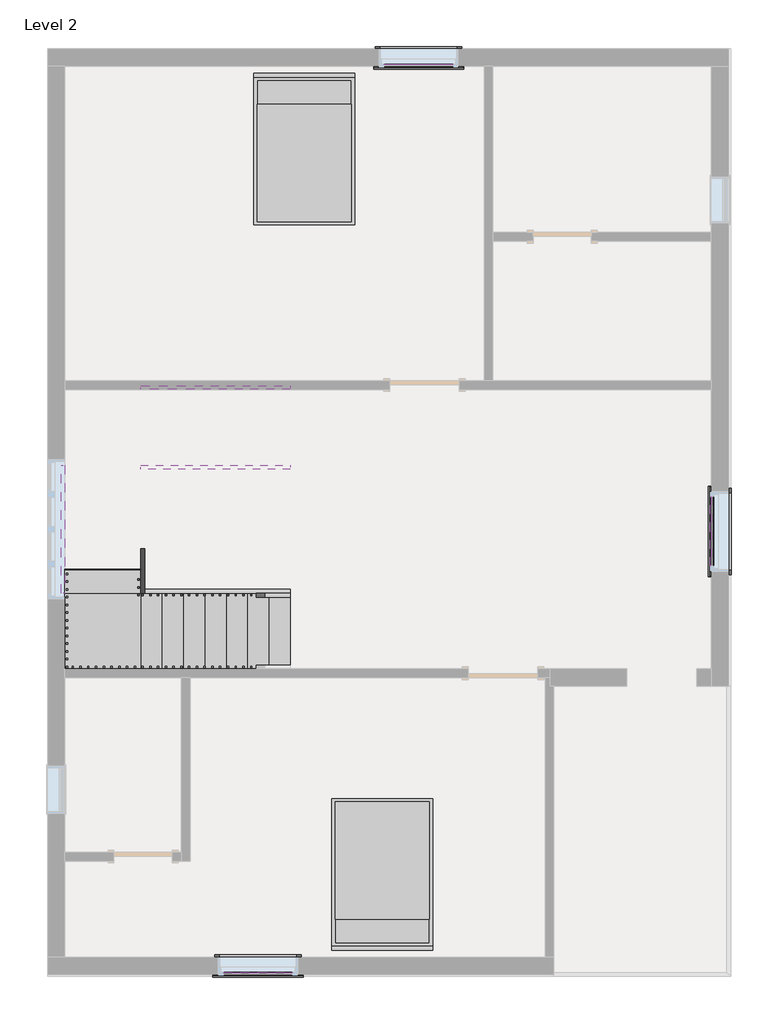
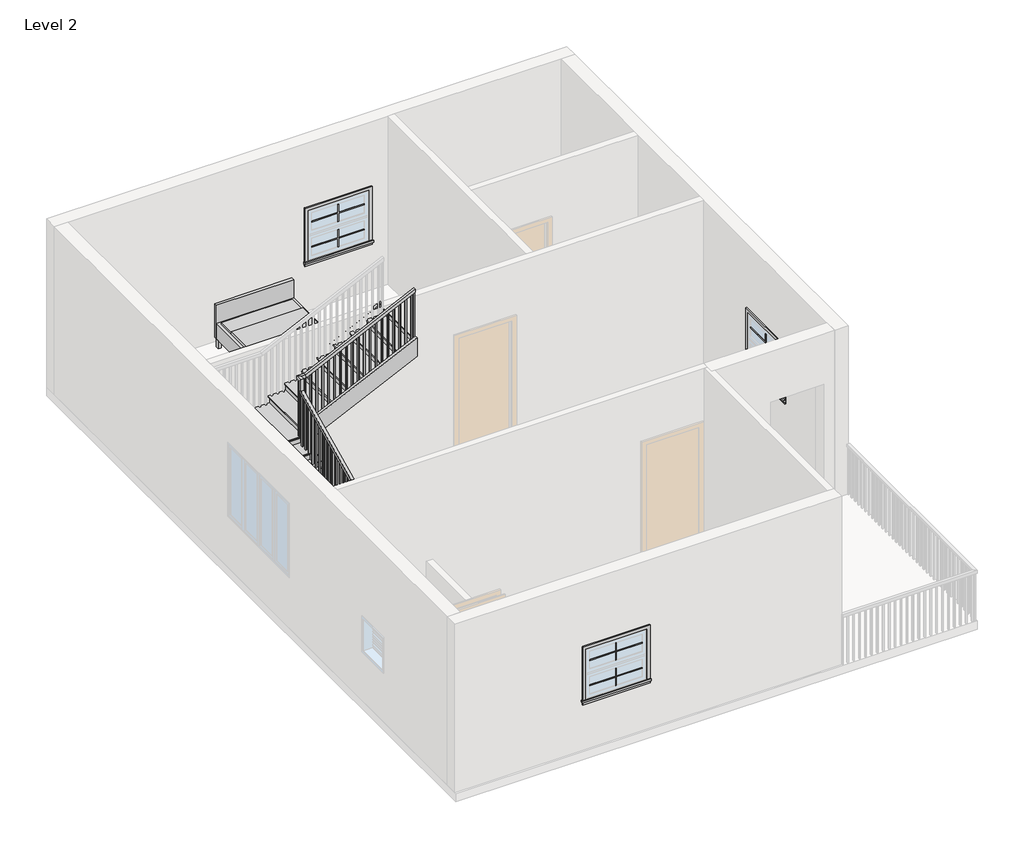
# One storey, part 3 of 3: 12 proxies, 6 members, 2 furniture elements, 1 railing, 1 stair flight.
"""IFC4 building model written with IfcOpenShell, lengths in millimetres."""

from ifc_helpers import new_model, si_unit, frame, origin, place, context, project, spatial, polyline, outline, extrude, faceted_brep, transform, mapped, element, save
from components import muntin_pattern_2x2_muntin_pattern_2x2_4e6d5dbc, muntin_pattern_2x2_muntin_pattern_2x2_9ec9cf3e, trim_window_exterior_flat_with_sill_79aa6636, trim_window_interior_flat_picture_frame_55a9d760, bed_17739_bed_17739_15c61121, stair_flight_9d362d5c

model = new_model("IFC4")

# Units and contexts
model_context = context("Model", 3, world=origin())
ifc_project = project(units=[si_unit("LENGTHUNIT", "METRE", prefix="MILLI")], contexts=[model_context])

# Site, building, storey
site = spatial("IfcSite", under=ifc_project)
building = spatial("IfcBuilding", under=site)
storey = spatial("IfcBuildingStorey", under=building, Name="Level 2", Elevation=3048.0)

# Proxies
placement = place(None, origin())
muntin_pattern_2x2_muntin_pattern_2x2_shape = muntin_pattern_2x2_muntin_pattern_2x2_4e6d5dbc(model_context)
element("IfcBuildingElementProxy", 1, Name="Muntin Pattern_2x2 : Muntin Pattern_2x2", ObjectType="Muntin Pattern_2x2 : Muntin Pattern_2x2", at=placement, inside=storey, context=model_context, shape_type="MappedRepresentation", body=[
    mapped(muntin_pattern_2x2_muntin_pattern_2x2_shape, transform((-20188.9789184, -5109.4149287, 4489.45), x_axis=(-1.0, 0.0, 0.0), y_axis=(0.0, -1.0, 0.0), z_axis=(0.0, 0.0, 1.0))),
])
element("IfcBuildingElementProxy", 2, Name="Muntin Pattern_2x2 : Muntin Pattern_2x2", ObjectType="Muntin Pattern_2x2 : Muntin Pattern_2x2", at=placement, inside=storey, context=model_context, shape_type="MappedRepresentation", body=[
    mapped(muntin_pattern_2x2_muntin_pattern_2x2_shape, transform((-14248.5539184, 681.7850713, 4489.45), x_axis=(0.0, 1.0, 0.0), y_axis=(-1.0, 0.0, 0.0), z_axis=(0.0, 0.0, 1.0))),
])
element("IfcBuildingElementProxy", 3, Name="Muntin Pattern_2x2 : Muntin Pattern_2x2", ObjectType="Muntin Pattern_2x2 : Muntin Pattern_2x2", at=placement, inside=storey, context=model_context, shape_type="MappedRepresentation", body=[
    mapped(muntin_pattern_2x2_muntin_pattern_2x2_shape, transform((-18087.1289184, 6777.7850713, 4489.45), x_axis=(-1.0, 0.0, 0.0), y_axis=(0.0, -1.0, 0.0), z_axis=(0.0, 0.0, 1.0))),
])
muntin_pattern_2x2_muntin_pattern_2x2_2_shape = muntin_pattern_2x2_muntin_pattern_2x2_9ec9cf3e(model_context)
element("IfcBuildingElementProxy", 4, Name="Muntin Pattern_2x2 : Muntin Pattern_2x2", ObjectType="Muntin Pattern_2x2 : Muntin Pattern_2x2", at=placement, inside=storey, context=model_context, shape_type="MappedRepresentation", body=[
    mapped(muntin_pattern_2x2_muntin_pattern_2x2_2_shape, transform((-20188.9789184, -5109.4149287, 4032.25), x_axis=(-1.0, 0.0, 0.0), y_axis=(0.0, -1.0, 0.0), z_axis=(0.0, 0.0, 1.0))),
])
element("IfcBuildingElementProxy", 5, Name="Muntin Pattern_2x2 : Muntin Pattern_2x2", ObjectType="Muntin Pattern_2x2 : Muntin Pattern_2x2", at=placement, inside=storey, context=model_context, shape_type="MappedRepresentation", body=[
    mapped(muntin_pattern_2x2_muntin_pattern_2x2_2_shape, transform((-14248.5539184, 681.7850713, 4032.25), x_axis=(0.0, 1.0, 0.0), y_axis=(-1.0, 0.0, 0.0), z_axis=(0.0, 0.0, 1.0))),
])
element("IfcBuildingElementProxy", 6, Name="Muntin Pattern_2x2 : Muntin Pattern_2x2", ObjectType="Muntin Pattern_2x2 : Muntin Pattern_2x2", at=placement, inside=storey, context=model_context, shape_type="MappedRepresentation", body=[
    mapped(muntin_pattern_2x2_muntin_pattern_2x2_2_shape, transform((-18087.1289184, 6777.7850713, 4032.25), x_axis=(-1.0, 0.0, 0.0), y_axis=(0.0, -1.0, 0.0), z_axis=(0.0, 0.0, 1.0))),
])
trim_window_exterior_flat_with_sill_shape = trim_window_exterior_flat_with_sill_79aa6636(model_context)
element("IfcBuildingElementProxy", 7, Name="Trim-Window-Exterior-Flat : with Sill", ObjectType="Trim-Window-Exterior-Flat : with Sill", at=placement, inside=storey, context=model_context, shape_type="MappedRepresentation", body=[
    mapped(trim_window_exterior_flat_with_sill_shape, transform((-20188.9789184, -5118.9399287, 4876.8), x_axis=(1.0, 0.0, 0.0), y_axis=(0.0, 0.0, 1.0), z_axis=(0.0, -1.0, 0.0))),
])
element("IfcBuildingElementProxy", 8, Name="Trim-Window-Exterior-Flat : with Sill", ObjectType="Trim-Window-Exterior-Flat : with Sill", at=placement, inside=storey, context=model_context, shape_type="MappedRepresentation", body=[
    mapped(trim_window_exterior_flat_with_sill_shape, transform((-14258.0789184, 681.7850713, 4876.8), x_axis=(0.0, -1.0, 0.0), y_axis=(0.0, 0.0, 1.0), z_axis=(-1.0, 0.0, 0.0))),
])
element("IfcBuildingElementProxy", 9, Name="Trim-Window-Exterior-Flat : with Sill", ObjectType="Trim-Window-Exterior-Flat : with Sill", at=placement, inside=storey, context=model_context, shape_type="MappedRepresentation", body=[
    mapped(trim_window_exterior_flat_with_sill_shape, transform((-18087.1289184, 6768.2600713, 4876.8), x_axis=(1.0, 0.0, 0.0), y_axis=(0.0, 0.0, 1.0), z_axis=(0.0, -1.0, 0.0))),
])
trim_window_interior_flat_picture_frame_shape = trim_window_interior_flat_picture_frame_55a9d760(model_context)
element("IfcBuildingElementProxy", 10, Name="Trim-Window-Interior-Flat : Picture Frame", ObjectType="Trim-Window-Interior-Flat : Picture Frame", at=placement, inside=storey, context=model_context, shape_type="MappedRepresentation", body=[
    mapped(trim_window_interior_flat_picture_frame_shape, transform((-20188.9789184, -4890.3399287, 4876.8), x_axis=(-1.0, 0.0, 0.0), y_axis=(0.0, 0.0, 1.0), z_axis=(0.0, 1.0, 0.0))),
])
element("IfcBuildingElementProxy", 11, Name="Trim-Window-Interior-Flat : Picture Frame", ObjectType="Trim-Window-Interior-Flat : Picture Frame", at=placement, inside=storey, context=model_context, shape_type="MappedRepresentation", body=[
    mapped(trim_window_interior_flat_picture_frame_shape, transform((-14029.4789184, 681.7850713, 4876.8), x_axis=(0.0, 1.0, 0.0), y_axis=(0.0, 0.0, 1.0), z_axis=(1.0, 0.0, 0.0))),
])
element("IfcBuildingElementProxy", 12, Name="Trim-Window-Interior-Flat : Picture Frame", ObjectType="Trim-Window-Interior-Flat : Picture Frame", at=placement, inside=storey, context=model_context, shape_type="MappedRepresentation", body=[
    mapped(trim_window_interior_flat_picture_frame_shape, transform((-18087.1289184, 6996.8600713, 4876.8), x_axis=(-1.0, 0.0, 0.0), y_axis=(0.0, 0.0, 1.0), z_axis=(0.0, 1.0, 0.0))),
])

# Furniture
bed_17739_bed_17739_shape = bed_17739_bed_17739_15c61121(model_context)
element("IfcFurniture", 13, ObjectType="Bed_17739 : Bed_17739", at=placement, inside=storey, context=model_context, shape_type="MappedRepresentation", body=[
    mapped(bed_17739_bed_17739_shape, transform((-18563.3789184, -3785.4399287, 3048.0), x_axis=(-1.0, 0.0, 0.0), y_axis=(0.0, -1.0, 0.0), z_axis=(0.0, 0.0, 1.0))),
])
element("IfcFurniture", 14, ObjectType="Bed_17739 : Bed_17739", at=placement, inside=storey, context=model_context, shape_type="MappedRepresentation", body=[
    mapped(bed_17739_bed_17739_shape, transform((-19585.7289184, 5663.3600713, 3048.0), x_axis=(1.0, 0.0, 0.0), y_axis=(0.0, 1.0, 0.0), z_axis=(0.0, 0.0, 1.0))),
])

# Members
element("IfcMember", 15, ObjectType="Stringer - 2\" Width", at=placement, inside=storey, context=model_context, shape_type="SweptSolid", body=[
    extrude(outline(polyline([(3048.0, -19769.8789184), (3249.2074226, -19769.8789184), (3839.5315333, -21014.4789184), (3839.5315333, -21725.7197387), (3048.0, -20056.9074227), (3048.0, -19769.8789184)])), frame((0.0, -1169.2399287, 0.0), z_axis=(0.0, 1.0, 0.0), x_axis=(0.0, 0.0, 1.0)), (0.0, 0.0, 1.0), 50.8),
])
element("IfcMember", 16, ObjectType="Stringer - 2\" Width", at=placement, inside=storey, context=model_context, shape_type="SweptSolid", body=[
    extrude(outline(polyline([(-127.880749, 4309.3619743), (837.3600713, 4767.1837072), (1548.6008915, 4767.1837072), (583.3600713, 4309.3619743), (-127.880749, 4309.3619743)])), frame((-22767.0789184, 0.0, 0.0), z_axis=(1.0, 0.0, 0.0), x_axis=(0.0, 1.0, 0.0)), (0.0, 0.0, 1.0), 50.8),
])
element("IfcMember", 17, ObjectType="Stringer - 2\" Width", at=placement, inside=storey, context=model_context, shape_type="SweptSolid", body=[
    extrude(outline(polyline([(5237.0141482, -21014.4789184), (5827.3382589, -19769.8789184), (6164.6856835, -19769.8789184), (5237.0141482, -21725.7197387), (5237.0141482, -21014.4789184)])), frame((0.0, 2539.1600713, 0.0), z_axis=(0.0, 1.0, 0.0), x_axis=(0.0, 0.0, 1.0)), (0.0, 0.0, 1.0), 50.8),
])
element("IfcMember", 18, ObjectType="Stringer - 2\" Width", at=placement, inside=storey, context=model_context, shape_type="SweptSolid", body=[
    extrude(outline(polyline([(3048.0, -19769.8789184), (3249.2074226, -19769.8789184), (4152.7647349, -21674.8789184), (3815.4173103, -21674.8789184), (3048.0, -20056.9074227), (3048.0, -19769.8789184)])), frame((0.0, -127.8399287, 0.0), z_axis=(0.0, 1.0, 0.0), x_axis=(0.0, 0.0, 1.0)), (0.0, 0.0, 1.0), 50.8),
])
element("IfcMember", 19, ObjectType="Stringer - 2\" Width", at=placement, inside=storey, context=model_context, shape_type="SweptSolid", body=[
    extrude(outline(polyline([(-127.8399287, 3972.033911), (-127.8399287, 4309.3813357), (1497.7600713, 5080.4169088), (1497.7600713, 4743.0694842), (-127.8399287, 3972.033911)])), frame((-21725.6789184, 0.0, 0.0), z_axis=(1.0, 0.0, 0.0), x_axis=(0.0, 1.0, 0.0)), (0.0, 0.0, 1.0), 50.8),
])
element("IfcMember", 20, ObjectType="Stringer - 2\" Width", at=placement, inside=storey, context=model_context, shape_type="SweptSolid", body=[
    extrude(outline(polyline([(5237.0335096, -21725.6789184), (4899.686085, -21725.6789184), (5827.3382589, -19769.8789184), (6164.6856835, -19769.8789184), (5237.0335096, -21725.6789184)])), frame((0.0, 1497.7600713, 0.0), z_axis=(0.0, 1.0, 0.0), x_axis=(0.0, 0.0, 1.0)), (0.0, 0.0, 1.0), 50.8),
])

# Railing
element("IfcRailing", 21, ObjectType="Handrail - Rectangular", at=placement, inside=storey, context=model_context, shape_type="SolidModel", body=[
    faceted_brep([(-19769.8789184, -178.6399287, 4094.9217391), (-19769.8789184, -178.6399287, 4038.6971684), (-19769.8789184, -127.8399287, 4038.6971684), (-19769.8789184, -127.8399287, 4094.9217391), (-21649.4789184, -178.6399287, 4986.4316206), (-21700.2789184, -178.6399287, 4954.3019114), (-21700.2789184, -127.8399287, 4954.3019114), (-21649.4789184, -127.8399287, 4986.4316206), (-21776.4789184, -40.2031254, 5140.4379447), (-21776.4789184, -51.6399287, 5191.2379447), (-21776.4789184, 1472.3600713, 5914.0837945), (-21776.4789184, 1523.1600713, 5881.9540854), (-21725.6789184, -40.2031254, 5140.4379447), (-21725.6789184, 1523.1600713, 5881.9540854), (-21725.6789184, -51.6399287, 5191.2379447), (-21725.6789184, 1472.3600713, 5914.0837945), (-19769.8789184, 1599.3600713, 7010.4), (-19769.8789184, 1548.5600713, 7010.4), (-19769.8789184, 1548.5600713, 6954.1754292), (-19769.8789184, 1599.3600713, 6954.1754292), (-21638.0421151, 1599.3600713, 6068.0901186), (-21649.4789184, 1599.3600713, 6118.8901186), (-21638.0421151, 1548.5600713, 6068.0901186), (-21649.4789184, 1548.5600713, 6118.8901186), (-21649.4789184, -178.6399287, 5191.2379447), (-21700.2789184, -178.6399287, 5140.4379447), (-21700.2789184, -127.8399287, 5140.4379447), (-21649.4789184, -127.8399287, 5191.2379447), (-21776.4789184, -178.6399287, 5191.2379447), (-21776.4789184, -178.6399287, 5140.4379447), (-21725.6789184, -127.8399287, 5140.4379447), (-21725.6789184, -127.8399287, 5191.2379447), (-21776.4789184, 1472.3600713, 6118.8901186), (-21776.4789184, 1523.1600713, 6068.0901186), (-21725.6789184, 1523.1600713, 6068.0901186), (-21725.6789184, 1472.3600713, 6118.8901186), (-21776.4789184, 1599.3600713, 6118.8901186), (-21776.4789184, 1599.3600713, 6068.0901186), (-21725.6789184, 1548.5600713, 6068.0901186), (-21725.6789184, 1548.5600713, 6118.8901186)], [[[0, 1, 2, 3]], [[1, 0, 4, 5]], [[2, 1, 5, 6]], [[3, 2, 6, 7]], [[0, 3, 7, 4]], [[8, 9, 10, 11]], [[12, 8, 11, 13]], [[14, 12, 13, 15]], [[9, 14, 15, 10]], [[16, 17, 18, 19]], [[20, 21, 16, 19]], [[22, 20, 19, 18]], [[23, 22, 18, 17]], [[21, 23, 17, 16]], [[5, 4, 24, 25]], [[6, 5, 25, 26]], [[7, 6, 26, 27]], [[4, 7, 27, 24]], [[25, 24, 28, 29]], [[26, 25, 29, 30]], [[27, 26, 30, 31]], [[24, 27, 31, 28]], [[29, 28, 9, 8]], [[30, 29, 8, 12]], [[31, 30, 12, 14]], [[28, 31, 14, 9]], [[11, 10, 32, 33]], [[13, 11, 33, 34]], [[15, 13, 34, 35]], [[10, 15, 35, 32]], [[33, 32, 36, 37]], [[34, 33, 37, 38]], [[35, 34, 38, 39]], [[32, 35, 39, 36]], [[37, 36, 21, 20]], [[38, 37, 20, 22]], [[39, 38, 22, 23]], [[36, 39, 23, 21]]]),
    extrude(outline(polyline([(6934.5983541, -19811.1539184), (6925.562781, -19830.2039184), (5963.4782609, -19830.2039184), (5963.4782609, -19811.1539184), (6934.5983541, -19811.1539184)])), frame((0.0, 1564.4350713, 0.0), z_axis=(0.0, 1.0, 0.0), x_axis=(0.0, 0.0, 1.0)), (0.0, 0.0, 1.0), 19.05),
    extrude(outline(polyline([(6886.4086308, -19912.7539184), (6877.3730577, -19931.8039184), (5963.4782609, -19931.8039184), (5963.4782609, -19912.7539184), (6886.4086308, -19912.7539184)])), frame((0.0, 1564.4350713, 0.0), z_axis=(0.0, 1.0, 0.0), x_axis=(0.0, 0.0, 1.0)), (0.0, 0.0, 1.0), 19.05),
    extrude(outline(polyline([(6838.2189075, -20014.3539184), (6829.1833344, -20033.4039184), (5963.4782609, -20033.4039184), (5963.4782609, -20014.3539184), (6838.2189075, -20014.3539184)])), frame((0.0, 1564.4350713, 0.0), z_axis=(0.0, 1.0, 0.0), x_axis=(0.0, 0.0, 1.0)), (0.0, 0.0, 1.0), 19.05),
    extrude(outline(polyline([(6790.0291842, -20115.9539184), (6780.993611, -20135.0039184), (5830.9565217, -20135.0039184), (5830.9565217, -20115.9539184), (6790.0291842, -20115.9539184)])), frame((0.0, 1564.4350713, 0.0), z_axis=(0.0, 1.0, 0.0), x_axis=(0.0, 0.0, 1.0)), (0.0, 0.0, 1.0), 19.05),
    extrude(outline(polyline([(6741.8394608, -20217.5539184), (6732.8038877, -20236.6039184), (5830.9565217, -20236.6039184), (5830.9565217, -20217.5539184), (6741.8394608, -20217.5539184)])), frame((0.0, 1564.4350713, 0.0), z_axis=(0.0, 1.0, 0.0), x_axis=(0.0, 0.0, 1.0)), (0.0, 0.0, 1.0), 19.05),
    extrude(outline(polyline([(6693.6497375, -20319.1539184), (6684.6141644, -20338.2039184), (5830.9565217, -20338.2039184), (5830.9565217, -20319.1539184), (6693.6497375, -20319.1539184)])), frame((0.0, 1564.4350713, 0.0), z_axis=(0.0, 1.0, 0.0), x_axis=(0.0, 0.0, 1.0)), (0.0, 0.0, 1.0), 19.05),
    extrude(outline(polyline([(6645.4600142, -20420.7539184), (6636.4244411, -20439.8039184), (5698.4347826, -20439.8039184), (5698.4347826, -20420.7539184), (6645.4600142, -20420.7539184)])), frame((0.0, 1564.4350713, 0.0), z_axis=(0.0, 1.0, 0.0), x_axis=(0.0, 0.0, 1.0)), (0.0, 0.0, 1.0), 19.05),
    extrude(outline(polyline([(6597.2702909, -20522.3539184), (6588.2347178, -20541.4039184), (5698.4347826, -20541.4039184), (5698.4347826, -20522.3539184), (6597.2702909, -20522.3539184)])), frame((0.0, 1564.4350713, 0.0), z_axis=(0.0, 1.0, 0.0), x_axis=(0.0, 0.0, 1.0)), (0.0, 0.0, 1.0), 19.05),
    extrude(outline(polyline([(6549.0805676, -20623.9539184), (6540.0449944, -20643.0039184), (5565.9130435, -20643.0039184), (5565.9130435, -20623.9539184), (6549.0805676, -20623.9539184)])), frame((0.0, 1564.4350713, 0.0), z_axis=(0.0, 1.0, 0.0), x_axis=(0.0, 0.0, 1.0)), (0.0, 0.0, 1.0), 19.05),
    extrude(outline(polyline([(6500.8908442, -20725.5539184), (6491.8552711, -20744.6039184), (5565.9130435, -20744.6039184), (5565.9130435, -20725.5539184), (6500.8908442, -20725.5539184)])), frame((0.0, 1564.4350713, 0.0), z_axis=(0.0, 1.0, 0.0), x_axis=(0.0, 0.0, 1.0)), (0.0, 0.0, 1.0), 19.05),
    extrude(outline(polyline([(6452.7011209, -20827.1539184), (6443.6655478, -20846.2039184), (5565.9130435, -20846.2039184), (5565.9130435, -20827.1539184), (6452.7011209, -20827.1539184)])), frame((0.0, 1564.4350713, 0.0), z_axis=(0.0, 1.0, 0.0), x_axis=(0.0, 0.0, 1.0)), (0.0, 0.0, 1.0), 19.05),
    extrude(outline(polyline([(6404.5113976, -20928.7539184), (6395.4758245, -20947.8039184), (5433.3913043, -20947.8039184), (5433.3913043, -20928.7539184), (6404.5113976, -20928.7539184)])), frame((0.0, 1564.4350713, 0.0), z_axis=(0.0, 1.0, 0.0), x_axis=(0.0, 0.0, 1.0)), (0.0, 0.0, 1.0), 19.05),
    extrude(outline(polyline([(6356.3216743, -21030.3539184), (6347.2861012, -21049.4039184), (5433.3913043, -21049.4039184), (5433.3913043, -21030.3539184), (6356.3216743, -21030.3539184)])), frame((0.0, 1564.4350713, 0.0), z_axis=(0.0, 1.0, 0.0), x_axis=(0.0, 0.0, 1.0)), (0.0, 0.0, 1.0), 19.05),
    extrude(outline(polyline([(6308.131951, -21131.9539184), (6299.0963778, -21151.0039184), (5433.3913043, -21151.0039184), (5433.3913043, -21131.9539184), (6308.131951, -21131.9539184)])), frame((0.0, 1564.4350713, 0.0), z_axis=(0.0, 1.0, 0.0), x_axis=(0.0, 0.0, 1.0)), (0.0, 0.0, 1.0), 19.05),
    extrude(outline(polyline([(6259.9422276, -21233.5539184), (6250.9066545, -21252.6039184), (5300.8695652, -21252.6039184), (5300.8695652, -21233.5539184), (6259.9422276, -21233.5539184)])), frame((0.0, 1564.4350713, 0.0), z_axis=(0.0, 1.0, 0.0), x_axis=(0.0, 0.0, 1.0)), (0.0, 0.0, 1.0), 19.05),
    extrude(outline(polyline([(6211.7525043, -21335.1539184), (6202.7169312, -21354.2039184), (5300.8695652, -21354.2039184), (5300.8695652, -21335.1539184), (6211.7525043, -21335.1539184)])), frame((0.0, 1564.4350713, 0.0), z_axis=(0.0, 1.0, 0.0), x_axis=(0.0, 0.0, 1.0)), (0.0, 0.0, 1.0), 19.05),
    extrude(outline(polyline([(6163.562781, -21436.7539184), (6154.5272079, -21455.8039184), (5300.8695652, -21455.8039184), (5300.8695652, -21436.7539184), (6163.562781, -21436.7539184)])), frame((0.0, 1564.4350713, 0.0), z_axis=(0.0, 1.0, 0.0), x_axis=(0.0, 0.0, 1.0)), (0.0, 0.0, 1.0), 19.05),
    extrude(outline(polyline([(6115.3730577, -21538.3539184), (6106.3374846, -21557.4039184), (5168.3478261, -21557.4039184), (5168.3478261, -21538.3539184), (6115.3730577, -21538.3539184)])), frame((0.0, 1564.4350713, 0.0), z_axis=(0.0, 1.0, 0.0), x_axis=(0.0, 0.0, 1.0)), (0.0, 0.0, 1.0), 19.05),
    extrude(outline(polyline([(6067.1833344, -21639.9539184), (6058.1477612, -21659.0039184), (5168.3478261, -21659.0039184), (5168.3478261, -21639.9539184), (6067.1833344, -21639.9539184)])), frame((0.0, 1564.4350713, 0.0), z_axis=(0.0, 1.0, 0.0), x_axis=(0.0, 0.0, 1.0)), (0.0, 0.0, 1.0), 19.05),
    extrude(outline(polyline([(1462.8350713, 5853.3414371), (1481.8850713, 5862.3770103), (1481.8850713, 4903.3043478), (1462.8350713, 4903.3043478), (1462.8350713, 5853.3414371)])), frame((-21760.6039184, 0.0, 0.0), z_axis=(1.0, 0.0, 0.0), x_axis=(0.0, 1.0, 0.0)), (0.0, 0.0, 1.0), 19.05),
    extrude(outline(polyline([(1361.2350713, 5805.1517138), (1380.2850713, 5814.1872869), (1380.2850713, 4903.3043478), (1361.2350713, 4903.3043478), (1361.2350713, 5805.1517138)])), frame((-21760.6039184, 0.0, 0.0), z_axis=(1.0, 0.0, 0.0), x_axis=(0.0, 1.0, 0.0)), (0.0, 0.0, 1.0), 19.05),
    extrude(outline(polyline([(1259.6350713, 5756.9619905), (1278.6850713, 5765.9975636), (1278.6850713, 4903.3043478), (1259.6350713, 4903.3043478), (1259.6350713, 5756.9619905)])), frame((-21760.6039184, 0.0, 0.0), z_axis=(1.0, 0.0, 0.0), x_axis=(0.0, 1.0, 0.0)), (0.0, 0.0, 1.0), 19.05),
    extrude(outline(polyline([(1158.0350713, 5708.7722672), (1177.0850713, 5717.8078403), (1177.0850713, 4770.7826087), (1158.0350713, 4770.7826087), (1158.0350713, 5708.7722672)])), frame((-21760.6039184, 0.0, 0.0), z_axis=(1.0, 0.0, 0.0), x_axis=(0.0, 1.0, 0.0)), (0.0, 0.0, 1.0), 19.05),
    extrude(outline(polyline([(1056.4350713, 5660.5825439), (1075.4850713, 5669.618117), (1075.4850713, 4770.7826087), (1056.4350713, 4770.7826087), (1056.4350713, 5660.5825439)])), frame((-21760.6039184, 0.0, 0.0), z_axis=(1.0, 0.0, 0.0), x_axis=(0.0, 1.0, 0.0)), (0.0, 0.0, 1.0), 19.05),
    extrude(outline(polyline([(954.8350713, 5612.3928205), (973.8850713, 5621.4283937), (973.8850713, 4638.2608696), (954.8350713, 4638.2608696), (954.8350713, 5612.3928205)])), frame((-21760.6039184, 0.0, 0.0), z_axis=(1.0, 0.0, 0.0), x_axis=(0.0, 1.0, 0.0)), (0.0, 0.0, 1.0), 19.05),
    extrude(outline(polyline([(853.2350713, 5564.2030972), (872.2850713, 5573.2386703), (872.2850713, 4638.2608696), (853.2350713, 4638.2608696), (853.2350713, 5564.2030972)])), frame((-21760.6039184, 0.0, 0.0), z_axis=(1.0, 0.0, 0.0), x_axis=(0.0, 1.0, 0.0)), (0.0, 0.0, 1.0), 19.05),
    extrude(outline(polyline([(751.6350713, 5516.0133739), (770.6850713, 5525.048947), (770.6850713, 4638.2608696), (751.6350713, 4638.2608696), (751.6350713, 5516.0133739)])), frame((-21760.6039184, 0.0, 0.0), z_axis=(1.0, 0.0, 0.0), x_axis=(0.0, 1.0, 0.0)), (0.0, 0.0, 1.0), 19.05),
    extrude(outline(polyline([(650.0350713, 5467.8236506), (669.0850713, 5476.8592237), (669.0850713, 4505.7391304), (650.0350713, 4505.7391304), (650.0350713, 5467.8236506)])), frame((-21760.6039184, 0.0, 0.0), z_axis=(1.0, 0.0, 0.0), x_axis=(0.0, 1.0, 0.0)), (0.0, 0.0, 1.0), 19.05),
    extrude(outline(polyline([(548.4350713, 5419.6339273), (567.4850713, 5428.6695004), (567.4850713, 4505.7391304), (548.4350713, 4505.7391304), (548.4350713, 5419.6339273)])), frame((-21760.6039184, 0.0, 0.0), z_axis=(1.0, 0.0, 0.0), x_axis=(0.0, 1.0, 0.0)), (0.0, 0.0, 1.0), 19.05),
    extrude(outline(polyline([(446.8350713, 5371.4442039), (465.8850713, 5380.4797771), (465.8850713, 4505.7391304), (446.8350713, 4505.7391304), (446.8350713, 5371.4442039)])), frame((-21760.6039184, 0.0, 0.0), z_axis=(1.0, 0.0, 0.0), x_axis=(0.0, 1.0, 0.0)), (0.0, 0.0, 1.0), 19.05),
    extrude(outline(polyline([(345.2350713, 5323.2544806), (364.2850713, 5332.2900537), (364.2850713, 4373.2173913), (345.2350713, 4373.2173913), (345.2350713, 5323.2544806)])), frame((-21760.6039184, 0.0, 0.0), z_axis=(1.0, 0.0, 0.0), x_axis=(0.0, 1.0, 0.0)), (0.0, 0.0, 1.0), 19.05),
    extrude(outline(polyline([(243.6350713, 5275.0647573), (262.6850713, 5284.1003304), (262.6850713, 4373.2173913), (243.6350713, 4373.2173913), (243.6350713, 5275.0647573)])), frame((-21760.6039184, 0.0, 0.0), z_axis=(1.0, 0.0, 0.0), x_axis=(0.0, 1.0, 0.0)), (0.0, 0.0, 1.0), 19.05),
    extrude(outline(polyline([(142.0350713, 5226.875034), (161.0850713, 5235.9106071), (161.0850713, 4373.2173913), (142.0350713, 4373.2173913), (142.0350713, 5226.875034)])), frame((-21760.6039184, 0.0, 0.0), z_axis=(1.0, 0.0, 0.0), x_axis=(0.0, 1.0, 0.0)), (0.0, 0.0, 1.0), 19.05),
    extrude(outline(polyline([(40.4350713, 5178.6853107), (59.4850713, 5187.7208838), (59.4850713, 4240.6956522), (40.4350713, 4240.6956522), (40.4350713, 5178.6853107)])), frame((-21760.6039184, 0.0, 0.0), z_axis=(1.0, 0.0, 0.0), x_axis=(0.0, 1.0, 0.0)), (0.0, 0.0, 1.0), 19.05),
    extrude(outline(polyline([(-61.1649287, 5130.4955873), (-42.1149287, 5139.5311605), (-42.1149287, 4240.6956522), (-61.1649287, 4240.6956522), (-61.1649287, 5130.4955873)])), frame((-21760.6039184, 0.0, 0.0), z_axis=(1.0, 0.0, 0.0), x_axis=(0.0, 1.0, 0.0)), (0.0, 0.0, 1.0), 19.05),
    extrude(outline(polyline([(-21690.7539184, -143.7149287), (-21690.7539184, -162.7649287), (-21709.8039184, -162.7649287), (-21709.8039184, -143.7149287), (-21690.7539184, -143.7149287)])), frame((0.0, 0.0, 3975.6521739), z_axis=(0.0, 0.0, 1.0), x_axis=(1.0, 0.0, 0.0)), (0.0, 0.0, 1.0), 1164.7857708),
    extrude(outline(polyline([(4901.5944016, -21589.1539184), (4910.6299747, -21608.2039184), (3975.6521739, -21608.2039184), (3975.6521739, -21589.1539184), (4901.5944016, -21589.1539184)])), frame((0.0, -162.7649287, 0.0), z_axis=(0.0, 1.0, 0.0), x_axis=(0.0, 0.0, 1.0)), (0.0, 0.0, 1.0), 19.05),
    extrude(outline(polyline([(4853.4046782, -21487.5539184), (4862.4402514, -21506.6039184), (3975.6521739, -21506.6039184), (3975.6521739, -21487.5539184), (4853.4046782, -21487.5539184)])), frame((0.0, -162.7649287, 0.0), z_axis=(0.0, 1.0, 0.0), x_axis=(0.0, 0.0, 1.0)), (0.0, 0.0, 1.0), 19.05),
    extrude(outline(polyline([(4805.2149549, -21385.9539184), (4814.250528, -21405.0039184), (3843.1304348, -21405.0039184), (3843.1304348, -21385.9539184), (4805.2149549, -21385.9539184)])), frame((0.0, -162.7649287, 0.0), z_axis=(0.0, 1.0, 0.0), x_axis=(0.0, 0.0, 1.0)), (0.0, 0.0, 1.0), 19.05),
    extrude(outline(polyline([(4757.0252316, -21284.3539184), (4766.0608047, -21303.4039184), (3843.1304348, -21303.4039184), (3843.1304348, -21284.3539184), (4757.0252316, -21284.3539184)])), frame((0.0, -162.7649287, 0.0), z_axis=(0.0, 1.0, 0.0), x_axis=(0.0, 0.0, 1.0)), (0.0, 0.0, 1.0), 19.05),
    extrude(outline(polyline([(4708.8355083, -21182.7539184), (4717.8710814, -21201.8039184), (3843.1304348, -21201.8039184), (3843.1304348, -21182.7539184), (4708.8355083, -21182.7539184)])), frame((0.0, -162.7649287, 0.0), z_axis=(0.0, 1.0, 0.0), x_axis=(0.0, 0.0, 1.0)), (0.0, 0.0, 1.0), 19.05),
    extrude(outline(polyline([(4660.645785, -21081.1539184), (4669.6813581, -21100.2039184), (3710.6086957, -21100.2039184), (3710.6086957, -21081.1539184), (4660.645785, -21081.1539184)])), frame((0.0, -162.7649287, 0.0), z_axis=(0.0, 1.0, 0.0), x_axis=(0.0, 0.0, 1.0)), (0.0, 0.0, 1.0), 19.05),
    extrude(outline(polyline([(4612.4560616, -20979.5539184), (4621.4916348, -20998.6039184), (3710.6086957, -20998.6039184), (3710.6086957, -20979.5539184), (4612.4560616, -20979.5539184)])), frame((0.0, -162.7649287, 0.0), z_axis=(0.0, 1.0, 0.0), x_axis=(0.0, 0.0, 1.0)), (0.0, 0.0, 1.0), 19.05),
    extrude(outline(polyline([(4564.2663383, -20877.9539184), (4573.3019114, -20897.0039184), (3710.6086957, -20897.0039184), (3710.6086957, -20877.9539184), (4564.2663383, -20877.9539184)])), frame((0.0, -162.7649287, 0.0), z_axis=(0.0, 1.0, 0.0), x_axis=(0.0, 0.0, 1.0)), (0.0, 0.0, 1.0), 19.05),
    extrude(outline(polyline([(4516.076615, -20776.3539184), (4525.1121881, -20795.4039184), (3578.0869565, -20795.4039184), (3578.0869565, -20776.3539184), (4516.076615, -20776.3539184)])), frame((0.0, -162.7649287, 0.0), z_axis=(0.0, 1.0, 0.0), x_axis=(0.0, 0.0, 1.0)), (0.0, 0.0, 1.0), 19.05),
    extrude(outline(polyline([(4467.8868917, -20674.7539184), (4476.9224648, -20693.8039184), (3578.0869565, -20693.8039184), (3578.0869565, -20674.7539184), (4467.8868917, -20674.7539184)])), frame((0.0, -162.7649287, 0.0), z_axis=(0.0, 1.0, 0.0), x_axis=(0.0, 0.0, 1.0)), (0.0, 0.0, 1.0), 19.05),
    extrude(outline(polyline([(4419.6971684, -20573.1539184), (4428.7327415, -20592.2039184), (3445.5652174, -20592.2039184), (3445.5652174, -20573.1539184), (4419.6971684, -20573.1539184)])), frame((0.0, -162.7649287, 0.0), z_axis=(0.0, 1.0, 0.0), x_axis=(0.0, 0.0, 1.0)), (0.0, 0.0, 1.0), 19.05),
    extrude(outline(polyline([(4371.507445, -20471.5539184), (4380.5430182, -20490.6039184), (3445.5652174, -20490.6039184), (3445.5652174, -20471.5539184), (4371.507445, -20471.5539184)])), frame((0.0, -162.7649287, 0.0), z_axis=(0.0, 1.0, 0.0), x_axis=(0.0, 0.0, 1.0)), (0.0, 0.0, 1.0), 19.05),
    extrude(outline(polyline([(4323.3177217, -20369.9539184), (4332.3532948, -20389.0039184), (3445.5652174, -20389.0039184), (3445.5652174, -20369.9539184), (4323.3177217, -20369.9539184)])), frame((0.0, -162.7649287, 0.0), z_axis=(0.0, 1.0, 0.0), x_axis=(0.0, 0.0, 1.0)), (0.0, 0.0, 1.0), 19.05),
    extrude(outline(polyline([(4275.1279984, -20268.3539184), (4284.1635715, -20287.4039184), (3313.0434783, -20287.4039184), (3313.0434783, -20268.3539184), (4275.1279984, -20268.3539184)])), frame((0.0, -162.7649287, 0.0), z_axis=(0.0, 1.0, 0.0), x_axis=(0.0, 0.0, 1.0)), (0.0, 0.0, 1.0), 19.05),
    extrude(outline(polyline([(4226.9382751, -20166.7539184), (4235.9738482, -20185.8039184), (3313.0434783, -20185.8039184), (3313.0434783, -20166.7539184), (4226.9382751, -20166.7539184)])), frame((0.0, -162.7649287, 0.0), z_axis=(0.0, 1.0, 0.0), x_axis=(0.0, 0.0, 1.0)), (0.0, 0.0, 1.0), 19.05),
    extrude(outline(polyline([(4178.7485518, -20065.1539184), (4187.7841249, -20084.2039184), (3313.0434783, -20084.2039184), (3313.0434783, -20065.1539184), (4178.7485518, -20065.1539184)])), frame((0.0, -162.7649287, 0.0), z_axis=(0.0, 1.0, 0.0), x_axis=(0.0, 0.0, 1.0)), (0.0, 0.0, 1.0), 19.05),
    extrude(outline(polyline([(4130.5588284, -19963.5539184), (4139.5944016, -19982.6039184), (3180.5217391, -19982.6039184), (3180.5217391, -19963.5539184), (4130.5588284, -19963.5539184)])), frame((0.0, -162.7649287, 0.0), z_axis=(0.0, 1.0, 0.0), x_axis=(0.0, 0.0, 1.0)), (0.0, 0.0, 1.0), 19.05),
    extrude(outline(polyline([(4082.3691051, -19861.9539184), (4091.4046782, -19881.0039184), (3180.5217391, -19881.0039184), (3180.5217391, -19861.9539184), (4082.3691051, -19861.9539184)])), frame((0.0, -162.7649287, 0.0), z_axis=(0.0, 1.0, 0.0), x_axis=(0.0, 0.0, 1.0)), (0.0, 0.0, 1.0), 19.05),
    extrude(outline(polyline([(-21741.5539184, 1564.4350713), (-21760.6039184, 1564.4350713), (-21760.6039184, 1583.4850713), (-21741.5539184, 1583.4850713), (-21741.5539184, 1564.4350713)])), frame((0.0, 0.0, 5035.826087), z_axis=(0.0, 0.0, 1.0), x_axis=(1.0, 0.0, 0.0)), (0.0, 0.0, 1.0), 1032.2640316),
    extrude(outline(polyline([(-21741.5539184, -143.7149287), (-21741.5539184, -162.7649287), (-21760.6039184, -162.7649287), (-21760.6039184, -143.7149287), (-21741.5539184, -143.7149287)])), frame((0.0, 0.0, 4108.173913), z_axis=(0.0, 0.0, 1.0), x_axis=(1.0, 0.0, 0.0)), (0.0, 0.0, 1.0), 1032.2640316),
    extrude(outline(polyline([(6954.1754292, -19769.8789184), (6945.1398561, -19788.9289184), (5963.4782609, -19788.9289184), (5963.4782609, -19769.8789184), (6954.1754292, -19769.8789184)])), frame((0.0, 1564.4350713, 0.0), z_axis=(0.0, 1.0, 0.0), x_axis=(0.0, 0.0, 1.0)), (0.0, 0.0, 1.0), 19.05),
    extrude(outline(polyline([(4038.6971684, -19769.8789184), (4047.7327415, -19788.9289184), (3180.5217391, -19788.9289184), (3180.5217391, -19769.8789184), (4038.6971684, -19769.8789184)])), frame((0.0, -162.7649287, 0.0), z_axis=(0.0, 1.0, 0.0), x_axis=(0.0, 0.0, 1.0)), (0.0, 0.0, 1.0), 19.05),
])

# Stair flight
stair_flight_shape = stair_flight_9d362d5c(model_context)
element("IfcStairFlight", 22, ObjectType="2\" Tread 1\" Nosing 1/4\" Riser", at=placement, inside=storey, context=model_context, shape_type="MappedRepresentation", body=[
    mapped(stair_flight_shape, transform((0.0, 0.0, 0.0), x_axis=(1.0, 0.0, 0.0), y_axis=(0.0, 1.0, 0.0), z_axis=(0.0, 0.0, 1.0))),
])

save(model, "model.ifc")

# Revit data of these elements
# Type "Muntin Pattern_2x2 : Muntin Pattern_2x2"
#   Width [instance default] = 4' - 0"
#   Thickness = 0' - 0 1/2"
#   Height [instance default] = 4' - 0"
#   Distance = 0' - 0 3/4"
#   Interior Material [instance default] = none
#   Exterior Material [instance default] = none
#   Default Elevation = 0
# Type "Trim-Window-Exterior-Flat : with Sill"
#   Trim Width = 0' - 2 1/4"
#   Trim Thickness_Picture Frame = 0' - 1 1/4"
#   Trim Thickness_with Sill = 0' - 0 3/4"
#   Sill Thickness = 0' - 1 1/4"
#   Opening Width [instance default] = 2' - 0"
#   Opening Height [instance default] = 3' - 0"
#   Default Elevation = 4' - 0"
#   Sill = yes
#   Picture Frame = no
#   Trim Material [instance default] = none
# Type "Trim-Window-Interior-Flat : Picture Frame"
#   Trim Thickness_Picture Frame = 0' - 1 1/4"
#   Trim Width = 0' - 2 1/4"
#   Trim Thickness_with Sill = 0' - 0 3/4"
#   Sill Thickness = 0' - 1 1/4"
#   Opening Width [instance default] = 2' - 0"
#   Opening Height [instance default] = 3' - 0"
#   Default Elevation = 4' - 0"
#   Sill = no
#   Picture Frame = yes
#   Trim Material [instance default] = none
# Type "Bed_17739 : Bed_17739"
#   Default Elevation = 0
# Type "Handrail - Rectangular"
#   Assembly Code = "C2010400"
#   built-in parameter 1008612 = 0.0416667 (stored number, unit not read)
#   built-in parameter 1008611 = 0.0416667 (stored number, unit not read)
#   built-in parameter 1008609 = 0.333333 (stored number, unit not read)
#   built-in parameter 1008604 = 0.166667 (stored number, unit not read)
#   built-in parameter 1008603 = 0.166667 (stored number, unit not read)
#   Railing Height = 3' - 0"
#   built-in parameter 1008630 = 2
#   built-in parameter 1008610 = 2
#   built-in parameter 1008618 = Baluster - Square : 3/4"
# Elements 1, 2, 3 (IfcBuildingElementProxy, "Muntin Pattern_2x2 : Muntin Pattern_2x2")
#   Width = 2' - 11 1/2"
#   Height = 1' - 0 1/2"
#   Interior Material = Wood - Stained
#   Exterior Material = Clad - White
#   Phase Created = New Construction
#   Materials on its faces: "Clad - White", "Wood - Stained"
# Elements 4, 5, 6 (IfcBuildingElementProxy, "Muntin Pattern_2x2 : Muntin Pattern_2x2")
#   Width = 2' - 11 1/2"
#   Height = 1' - 0.49965"
#   Interior Material = Wood - Stained
#   Exterior Material = Clad - White
#   Phase Created = New Construction
#   Materials on its faces: "Clad - White", "Wood - Stained"
# Elements 7, 8, 9 (IfcBuildingElementProxy, "Trim-Window-Exterior-Flat : with Sill")
#   Opening Width = 3' - 5"
#   Opening Height = 3' - 0"
#   Trim Material = Clad - White
#   Phase Created = New Construction
#   Materials on its faces: "Clad - White"
# Elements 10, 11, 12 (IfcBuildingElementProxy, "Trim-Window-Interior-Flat : Picture Frame")
#   Opening Width = 3' - 5"
#   Opening Height = 3' - 0"
#   Trim Material = Wood - Stained
#   Phase Created = New Construction
#   Materials on its faces: "Wood - Stained"
# Elements 13, 14 (IfcFurniture, "Bed_17739 : Bed_17739")
#   Phase Created = New Construction
#   Materials on its faces: "legs", "sheets", "bed frame", "Blanket"
# Elements 15, 16, 17, 18, 19, 20 (IfcMember, "Stringer - 2\" Width")
#   Phase Created = New Construction
# Element 21 (IfcRailing, "Handrail - Rectangular")
#   Phase Created = New Construction
# Element 22 (IfcStairFlight, "2\" Tread 1\" Nosing 1/4\" Riser")
#   Phase Created = New Construction
# Materials
#   "Clad - White": class "Wood", colour RGB 242 242 238, transparency 0, Cost = 0
#   "Wood - Stained": class "Wood", colour RGB 224 178 126, transparency 0, Cost = 0
#   "legs": colour RGB 90 73 37, transparency 0, Cost = 0
#   "sheets": colour RGB 200 195 176, transparency 0, Cost = 0
#   "bed frame": colour RGB 90 73 37, transparency 0, Cost = 0
#   "Blanket": class "System", colour RGB 59 0 1, transparency 0, Cost = 0
